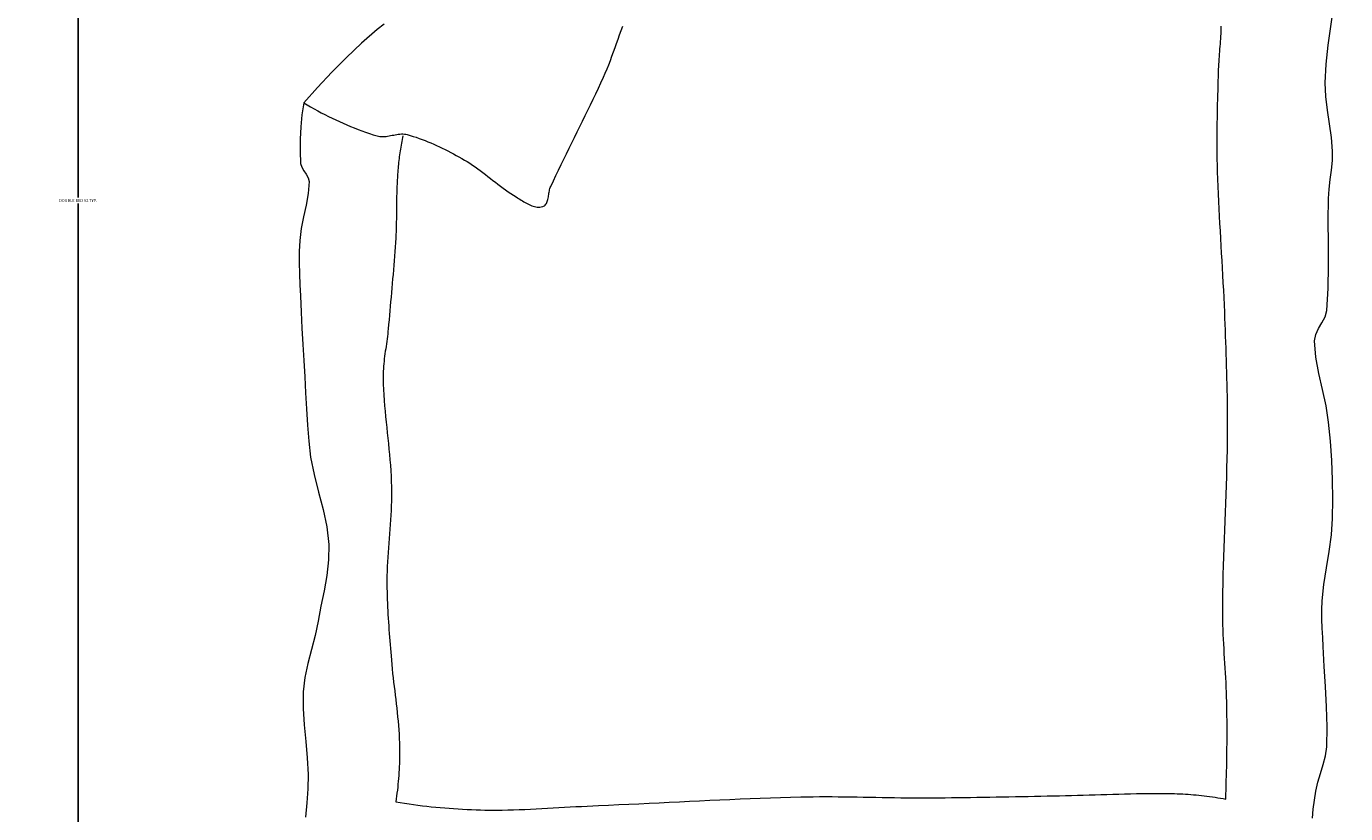
# Model space of a CAD drawing. Units: inches. Extents: x 1441 to 2460, y 1648 to 2683.
# Tile 23 of 35: x 1792 to 1874, y 2204 to 2253. Entities that reach past the tile are written whole.
import ezdxf

# ---------------------------------------------------------------- set-up
doc = ezdxf.new("R2010")
doc.units = ezdxf.units.IN
doc.layers.add('A-ANNO-DIMS', color=2, linetype='Continuous', lineweight=18)
doc.layers.add('A-FURN', color=8, linetype='Continuous', lineweight=15)
doc.styles.get("Standard").update_dxf_attribs({"font": 'arial.ttf'})
doc.dimstyles.get("Standard").update_dxf_attribs({"dimtxt": 0.18, "dimasz": 0.18, "dimexe": 0.18, "dimexo": 0.0625, "dimgap": 0.09, "dimtad": 0, "dimtih": 1, "dimtoh": 1, "dimdec": 4, "dimzin": 0, "dimdsep": 46, "dimtxsty": 'Standard', "dimcen": 0.09, "dimadec": 0, "dimazin": 0, "dimtfac": 1, "dimtdec": 4, "dimtofl": 0, "dimtmove": 0, "dimatfit": 3, "dimfxl": 1, "dimtolj": 1, "dimtzin": 0, "dimarcsym": 0})

# ---------------------------------------------------------------- blocks, each defined once
blk = doc.blocks.new('BED-DOUBLE-PLAN')
for p, q in [((64.222, 56.681), (64.382, 57.848)), ((5.285, 56.837), (4.851, 56.5)), ((20.05, 56.435), (20.15, 56.7)), ((57.394, 56.548), (57.398, 56.707)), ((64.06, 55.515), (64.222, 56.681)), ((4.851, 56.5), (3.888, 55.638)), ((19.761, 55.634), (19.856, 55.902)), ((19.856, 55.902), (19.952, 56.169)), ((19.952, 56.169), (20.05, 56.435)), ((57.353, 55.757), (57.363, 55.915)), ((57.363, 55.915), (57.373, 56.073)), ((57.373, 56.073), (57.382, 56.232)), ((57.382, 56.232), (57.389, 56.39)), ((57.389, 56.39), (57.394, 56.548)), ((3.888, 55.638), (2.949, 54.748)), ((19.474, 54.832), (19.571, 55.099)), ((19.571, 55.099), (19.666, 55.367)), ((19.666, 55.367), (19.761, 55.634)), ((57.291, 54.965), (57.304, 55.123)), ((57.304, 55.123), (57.316, 55.282)), ((57.316, 55.282), (57.329, 55.44)), ((57.329, 55.44), (57.341, 55.598)), ((57.341, 55.598), (57.353, 55.757)), ((63.929, 54.347), (64.06, 55.515)), ((2.949, 54.748), (2.036, 53.833)), ((19.169, 54.039), (19.274, 54.302)), ((19.274, 54.302), (19.375, 54.566)), ((19.375, 54.566), (19.474, 54.832)), ((57.239, 54.173), (57.247, 54.332)), ((57.247, 54.332), (57.257, 54.49)), ((57.257, 54.49), (57.268, 54.649)), ((57.268, 54.649), (57.279, 54.807)), ((57.279, 54.807), (57.291, 54.965)), ((63.863, 53.174), (63.929, 54.347)), ((2.036, 53.833), (1.148, 52.892)), ((18.788, 53.177), (18.945, 53.52)), ((18.945, 53.52), (19.059, 53.778)), ((19.059, 53.778), (19.169, 54.039)), ((57.21, 53.28), (57.218, 53.568)), ((57.218, 53.568), (57.227, 53.856)), ((57.227, 53.856), (57.232, 54.015)), ((57.232, 54.015), (57.239, 54.173)), ((1.148, 52.892), (0.288, 51.928)), ((18.468, 52.493), (18.629, 52.834)), ((18.629, 52.834), (18.788, 53.177)), ((57.186, 52.417), (57.194, 52.705)), ((57.194, 52.705), (57.202, 52.993)), ((57.202, 52.993), (57.21, 53.28)), ((63.897, 52.321), (63.863, 53.174)), ((0.288, 51.928), (0.178, 51.18)), ((0.288, 51.928), (0.502, 51.799)), ((0.502, 51.799), (0.719, 51.672)), ((17.979, 51.472), (18.143, 51.812)), ((18.143, 51.812), (18.306, 52.152)), ((18.306, 52.152), (18.468, 52.493)), ((57.164, 51.553), (57.171, 51.841)), ((57.171, 51.841), (57.178, 52.129)), ((57.178, 52.129), (57.186, 52.417)), ((64.002, 51.471), (63.897, 52.321)), ((0.178, 51.18), (0.104, 50.426)), ((0.719, 51.672), (0.936, 51.548)), ((0.936, 51.548), (1.156, 51.426)), ((1.156, 51.426), (1.377, 51.308)), ((1.377, 51.308), (1.6, 51.192)), ((1.6, 51.192), (1.824, 51.079)), ((1.824, 51.079), (2.05, 50.968)), ((2.05, 50.968), (2.277, 50.861)), ((17.648, 50.793), (17.814, 51.132)), ((17.814, 51.132), (17.979, 51.472)), ((57.147, 50.688), (57.152, 50.976)), ((57.152, 50.976), (57.158, 51.265)), ((57.158, 51.265), (57.164, 51.553)), ((64.135, 50.622), (64.002, 51.471)), ((0.104, 50.426), (0.065, 49.669)), ((2.277, 50.861), (2.505, 50.756)), ((2.505, 50.756), (2.735, 50.654)), ((2.735, 50.654), (2.966, 50.555)), ((2.966, 50.555), (3.198, 50.459)), ((3.198, 50.459), (3.432, 50.366)), ((3.432, 50.366), (3.666, 50.276)), ((3.666, 50.276), (3.901, 50.189)), ((3.901, 50.189), (4.138, 50.105)), ((4.138, 50.105), (4.375, 50.024)), ((17.147, 49.777), (17.314, 50.116)), ((17.314, 50.116), (17.481, 50.455)), ((17.481, 50.455), (17.648, 50.793)), ((57.138, 49.824), (57.14, 50.112)), ((57.14, 50.112), (57.143, 50.4)), ((57.143, 50.4), (57.147, 50.688)), ((64.256, 49.773), (64.135, 50.622)), ((0.065, 49.669), (0.062, 48.911)), ((4.375, 50.024), (4.613, 49.946)), ((4.613, 49.946), (4.852, 49.871)), ((4.852, 49.871), (4.943, 49.848)), ((4.943, 49.848), (5.034, 49.833)), ((5.034, 49.833), (5.127, 49.826)), ((5.127, 49.826), (5.22, 49.825)), ((5.22, 49.825), (5.314, 49.829)), ((5.314, 49.829), (5.409, 49.839)), ((5.409, 49.839), (5.504, 49.852)), ((5.504, 49.852), (5.6, 49.868)), ((5.6, 49.868), (5.695, 49.886)), ((5.695, 49.886), (5.791, 49.905)), ((5.791, 49.905), (5.887, 49.924)), ((5.887, 49.924), (5.983, 49.943)), ((5.983, 49.943), (6.079, 49.96)), ((6.079, 49.96), (6.174, 49.974)), ((6.174, 49.974), (6.269, 49.984)), ((6.269, 49.984), (6.363, 49.99)), ((6.347, 49.291), (6.326, 49.172)), ((6.368, 49.41), (6.347, 49.291)), ((6.363, 49.99), (6.457, 49.991)), ((6.39, 49.528), (6.368, 49.41)), ((6.412, 49.647), (6.39, 49.528)), ((6.436, 49.765), (6.412, 49.647)), ((6.46, 49.883), (6.436, 49.765)), ((6.457, 49.991), (6.55, 49.986)), ((6.55, 49.986), (6.643, 49.973)), ((6.643, 49.973), (6.734, 49.952)), ((6.734, 49.952), (6.921, 49.899)), ((6.921, 49.899), (7.107, 49.841)), ((7.107, 49.841), (7.292, 49.781)), ((7.292, 49.781), (7.476, 49.717)), ((7.476, 49.717), (7.659, 49.65)), ((7.659, 49.65), (7.841, 49.58)), ((7.841, 49.58), (8.022, 49.507)), ((8.022, 49.507), (8.202, 49.431)), ((8.202, 49.431), (8.381, 49.353)), ((8.381, 49.353), (8.56, 49.273)), ((8.56, 49.273), (8.737, 49.19)), ((16.813, 49.1), (16.98, 49.439)), ((16.98, 49.439), (17.147, 49.777)), ((57.137, 49.536), (57.138, 49.824)), ((57.137, 49.248), (57.137, 49.536)), ((64.322, 48.92), (64.256, 49.773)), ((0.062, 48.911), (0.095, 48.156)), ((6.221, 48.455), (6.207, 48.335)), ((6.237, 48.575), (6.221, 48.455)), ((6.253, 48.694), (6.237, 48.575)), ((6.27, 48.814), (6.253, 48.694)), ((6.288, 48.933), (6.27, 48.814)), ((6.307, 49.053), (6.288, 48.933)), ((6.326, 49.172), (6.307, 49.053)), ((8.737, 49.19), (8.913, 49.105)), ((8.913, 49.105), (9.088, 49.019)), ((9.088, 49.019), (9.263, 48.93)), ((9.263, 48.93), (9.436, 48.84)), ((9.436, 48.84), (9.609, 48.748)), ((9.609, 48.748), (9.781, 48.655)), ((9.781, 48.655), (9.952, 48.56)), ((9.952, 48.56), (10.122, 48.465)), ((10.122, 48.465), (10.291, 48.368)), ((16.481, 48.423), (16.647, 48.762)), ((16.647, 48.762), (16.813, 49.1)), ((57.139, 48.96), (57.137, 49.248)), ((57.142, 48.672), (57.139, 48.96)), ((57.147, 48.384), (57.142, 48.672)), ((64.311, 48.328), (64.322, 48.92)), ((0.095, 48.156), (0.161, 47.92)), ((0.161, 47.92), (0.294, 47.701)), ((0.294, 47.701), (0.446, 47.487)), ((6.146, 47.734), (6.136, 47.614)), ((6.156, 47.855), (6.146, 47.734)), ((6.168, 47.975), (6.156, 47.855)), ((6.18, 48.095), (6.168, 47.975)), ((6.193, 48.215), (6.18, 48.095)), ((6.207, 48.335), (6.193, 48.215)), ((10.291, 48.368), (10.462, 48.268)), ((10.462, 48.268), (10.629, 48.163)), ((10.629, 48.163), (10.794, 48.054)), ((10.794, 48.054), (10.957, 47.942)), ((10.957, 47.942), (11.118, 47.827)), ((11.118, 47.827), (11.277, 47.709)), ((11.277, 47.709), (11.435, 47.59)), ((15.987, 47.404), (16.151, 47.744)), ((16.151, 47.744), (16.315, 48.084)), ((16.315, 48.084), (16.481, 48.423)), ((57.153, 48.096), (57.147, 48.384)), ((57.167, 47.636), (57.153, 48.096)), ((57.182, 47.175), (57.167, 47.636)), ((64.185, 47.146), (64.258, 47.737)), ((64.258, 47.737), (64.311, 48.328)), ((0.446, 47.487), (0.571, 47.267)), ((0.62, 47.031), (0.562, 46.291)), ((0.571, 47.267), (0.62, 47.031)), ((6.095, 46.897), (6.087, 46.698)), ((6.104, 47.096), (6.095, 46.897)), ((6.114, 47.295), (6.104, 47.096)), ((6.127, 47.494), (6.114, 47.295)), ((6.136, 47.614), (6.127, 47.494)), ((11.435, 47.59), (11.593, 47.469)), ((11.593, 47.469), (11.749, 47.347)), ((11.749, 47.347), (11.905, 47.224)), ((11.905, 47.224), (12.061, 47.101)), ((12.061, 47.101), (12.218, 46.979)), ((12.218, 46.979), (12.374, 46.857)), ((12.374, 46.857), (12.532, 46.737)), ((15.663, 46.722), (15.824, 47.063)), ((15.824, 47.063), (15.987, 47.404)), ((57.2, 46.714), (57.182, 47.175)), ((64.117, 46.556), (64.185, 47.146)), ((0.562, 46.291), (0.434, 45.558)), ((6.072, 46.1), (6.069, 45.901)), ((6.076, 46.3), (6.072, 46.1)), ((6.081, 46.499), (6.076, 46.3)), ((6.087, 46.698), (6.081, 46.499)), ((12.532, 46.737), (12.691, 46.618)), ((12.691, 46.618), (12.851, 46.501)), ((12.851, 46.501), (13.012, 46.387)), ((13.012, 46.387), (13.176, 46.276)), ((13.176, 46.276), (13.342, 46.169)), ((13.342, 46.169), (13.511, 46.065)), ((13.511, 46.065), (13.587, 46.019)), ((13.587, 46.019), (13.664, 45.971)), ((15.486, 45.917), (15.502, 45.99)), ((15.502, 45.99), (15.515, 46.065)), ((15.515, 46.065), (15.527, 46.141)), ((15.527, 46.141), (15.539, 46.218)), ((15.539, 46.218), (15.551, 46.295)), ((15.551, 46.295), (15.564, 46.372)), ((15.564, 46.372), (15.578, 46.447)), ((15.578, 46.447), (15.595, 46.52)), ((15.595, 46.52), (15.614, 46.591)), ((15.614, 46.591), (15.636, 46.659)), ((15.636, 46.659), (15.663, 46.722)), ((57.22, 46.253), (57.2, 46.714)), ((57.241, 45.792), (57.22, 46.253)), ((64.074, 45.964), (64.117, 46.556)), ((0.434, 45.558), (0.277, 44.827)), ((6.062, 45.303), (6.06, 45.104)), ((6.064, 45.502), (6.062, 45.303)), ((6.067, 45.702), (6.064, 45.502)), ((6.069, 45.901), (6.067, 45.702)), ((13.664, 45.971), (13.742, 45.922)), ((13.742, 45.922), (13.822, 45.871)), ((13.822, 45.871), (13.902, 45.821)), ((13.902, 45.821), (13.983, 45.771)), ((13.983, 45.771), (14.065, 45.723)), ((14.065, 45.723), (14.147, 45.676)), ((14.147, 45.676), (14.231, 45.631)), ((14.231, 45.631), (14.314, 45.589)), ((14.314, 45.589), (14.398, 45.551)), ((14.398, 45.551), (14.483, 45.517)), ((14.483, 45.517), (14.567, 45.487)), ((14.567, 45.487), (14.652, 45.463)), ((14.652, 45.463), (14.737, 45.445)), ((14.737, 45.445), (14.822, 45.434)), ((14.822, 45.434), (14.907, 45.429)), ((14.907, 45.429), (14.992, 45.433)), ((14.992, 45.433), (15.076, 45.445)), ((15.076, 45.445), (15.16, 45.466)), ((15.16, 45.466), (15.221, 45.49)), ((15.221, 45.49), (15.274, 45.522)), ((15.274, 45.522), (15.32, 45.561)), ((15.32, 45.561), (15.36, 45.608)), ((15.36, 45.608), (15.394, 45.66)), ((15.394, 45.66), (15.423, 45.718)), ((15.423, 45.718), (15.448, 45.78)), ((15.448, 45.78), (15.468, 45.847)), ((15.468, 45.847), (15.486, 45.917)), ((57.264, 45.332), (57.241, 45.792)), ((57.289, 44.871), (57.264, 45.332)), ((64.052, 44.569), (64.074, 45.964)), ((0.277, 44.827), (0.13, 44.094)), ((6.05, 44.506), (6.045, 44.306)), ((6.054, 44.705), (6.05, 44.506)), ((6.057, 44.904), (6.054, 44.705)), ((6.06, 45.104), (6.057, 44.904)), ((57.314, 44.411), (57.289, 44.871)), ((57.34, 43.95), (57.314, 44.411)), ((64.063, 43.173), (64.052, 44.569)), ((0.13, 44.094), (0.035, 43.356)), ((6.022, 43.709), (6.011, 43.51)), ((6.031, 43.908), (6.022, 43.709)), ((6.039, 44.107), (6.031, 43.908)), ((6.045, 44.306), (6.039, 44.107)), ((57.367, 43.49), (57.34, 43.95)), ((0.035, 43.356), (0.002, 42.668)), ((5.975, 42.943), (5.955, 42.66)), ((5.993, 43.227), (5.975, 42.943)), ((6.011, 43.51), (5.993, 43.227)), ((57.394, 43.029), (57.367, 43.49)), ((57.42, 42.569), (57.394, 43.029)), ((64.074, 41.778), (64.063, 43.173)), ((0.002, 42.668), (0.002, 41.978)), ((0.002, 41.978), (0.023, 41.288)), ((5.914, 42.093), (5.892, 41.81)), ((5.935, 42.376), (5.914, 42.093)), ((5.955, 42.66), (5.935, 42.376)), ((57.447, 42.108), (57.42, 42.569)), ((57.474, 41.648), (57.447, 42.108)), ((0.023, 41.288), (0.053, 40.599)), ((5.846, 41.243), (5.822, 40.96)), ((5.869, 41.527), (5.846, 41.243)), ((5.892, 41.81), (5.869, 41.527)), ((57.499, 41.187), (57.474, 41.648)), ((57.524, 40.727), (57.499, 41.187)), ((64.051, 40.384), (64.074, 41.778)), ((0.053, 40.599), (0.083, 39.909)), ((5.774, 40.394), (5.749, 40.111)), ((5.798, 40.677), (5.774, 40.394)), ((5.822, 40.96), (5.798, 40.677)), ((57.548, 40.266), (57.524, 40.727)), ((57.57, 39.806), (57.548, 40.266)), ((63.96, 38.994), (64.051, 40.384)), ((0.083, 39.909), (0.124, 38.9)), ((5.698, 39.545), (5.673, 39.262)), ((5.724, 39.828), (5.698, 39.545)), ((5.749, 40.111), (5.724, 39.828)), ((57.59, 39.345), (57.57, 39.806)), ((0.124, 38.9), (0.172, 37.892)), ((5.621, 38.696), (5.596, 38.413)), ((5.647, 38.979), (5.621, 38.696)), ((5.673, 39.262), (5.647, 38.979)), ((57.609, 38.884), (57.59, 39.345)), ((57.623, 38.511), (57.609, 38.884)), ((63.663, 38.235), (63.855, 38.605)), ((63.855, 38.605), (63.96, 38.994)), ((0.172, 37.892), (0.227, 36.884)), ((5.545, 37.847), (5.53, 37.692)), ((5.57, 38.13), (5.545, 37.847)), ((5.596, 38.413), (5.57, 38.13)), ((57.637, 38.138), (57.623, 38.511)), ((57.652, 37.765), (57.637, 38.138)), ((63.274, 37.501), (63.447, 37.871)), ((63.447, 37.871), (63.663, 38.235)), ((5.453, 37.073), (5.432, 36.918)), ((5.474, 37.227), (5.453, 37.073)), ((5.494, 37.382), (5.474, 37.227)), ((5.513, 37.537), (5.494, 37.382)), ((5.53, 37.692), (5.513, 37.537)), ((57.666, 37.393), (57.652, 37.765)), ((57.68, 37.02), (57.666, 37.393)), ((57.693, 36.647), (57.68, 37.02)), ((63.206, 37.11), (63.274, 37.501)), ((63.291, 36.09), (63.206, 37.11)), ((0.227, 36.884), (0.286, 35.876)), ((5.324, 36.144), (5.304, 35.989)), ((5.344, 36.299), (5.324, 36.144)), ((5.366, 36.454), (5.344, 36.299)), ((5.388, 36.608), (5.366, 36.454)), ((5.41, 36.763), (5.388, 36.608)), ((5.432, 36.918), (5.41, 36.763)), ((57.706, 36.274), (57.693, 36.647)), ((57.718, 35.901), (57.706, 36.274)), ((0.286, 35.876), (0.348, 34.868)), ((5.245, 35.369), (5.236, 35.214)), ((5.256, 35.524), (5.245, 35.369)), ((5.27, 35.679), (5.256, 35.524)), ((5.287, 35.834), (5.27, 35.679)), ((5.304, 35.989), (5.287, 35.834)), ((57.73, 35.528), (57.718, 35.901)), ((57.741, 35.155), (57.73, 35.528)), ((63.474, 35.079), (63.291, 36.09)), ((0.348, 34.868), (0.404, 33.866)), ((5.23, 35.059), (5.228, 34.903)), ((5.228, 34.903), (5.229, 34.747)), ((5.229, 34.747), (5.239, 34.409)), ((5.236, 35.214), (5.23, 35.059)), ((57.751, 34.782), (57.741, 35.155)), ((57.761, 34.409), (57.751, 34.782)), ((63.703, 34.073), (63.474, 35.079)), ((0.404, 33.866), (0.456, 32.863)), ((5.239, 34.409), (5.254, 34.072)), ((5.254, 34.072), (5.274, 33.735)), ((5.274, 33.735), (5.297, 33.397)), ((57.769, 34.036), (57.761, 34.409)), ((57.776, 33.663), (57.769, 34.036)), ((63.921, 33.064), (63.703, 34.073)), ((0.456, 32.863), (0.516, 31.861)), ((5.297, 33.397), (5.324, 33.06)), ((5.324, 33.06), (5.354, 32.724)), ((57.782, 33.29), (57.776, 33.663)), ((57.787, 32.917), (57.782, 33.29)), ((57.79, 32.543), (57.787, 32.917)), ((64.075, 32.048), (63.921, 33.064)), ((5.354, 32.724), (5.386, 32.387)), ((5.386, 32.387), (5.42, 32.05)), ((5.42, 32.05), (5.455, 31.714)), ((57.792, 32.17), (57.79, 32.543)), ((57.792, 31.797), (57.792, 32.17)), ((64.186, 30.851), (64.075, 32.048)), ((0.516, 31.861), (0.599, 30.861)), ((5.455, 31.714), (5.491, 31.377)), ((5.491, 31.377), (5.526, 31.04)), ((57.785, 30.869), (57.79, 31.424)), ((57.79, 31.424), (57.792, 31.797)), ((0.599, 30.861), (0.719, 29.866)), ((5.526, 31.04), (5.561, 30.704)), ((5.561, 30.704), (5.595, 30.367)), ((57.777, 30.314), (57.785, 30.869)), ((64.273, 29.652), (64.186, 30.851)), ((0.719, 29.866), (0.929, 28.772)), ((5.595, 30.367), (5.627, 30.03)), ((5.627, 30.03), (5.656, 29.694)), ((5.656, 29.694), (5.683, 29.357)), ((57.751, 29.204), (57.765, 29.759)), ((57.765, 29.759), (57.777, 30.314)), ((64.329, 28.45), (64.273, 29.652)), ((0.929, 28.772), (1.205, 27.689)), ((5.683, 29.357), (5.706, 29.019)), ((5.706, 29.019), (5.725, 28.682)), ((57.735, 28.65), (57.751, 29.204)), ((5.725, 28.682), (5.74, 28.344)), ((5.74, 28.344), (5.749, 28.007)), ((5.749, 28.007), (5.752, 27.715)), ((57.698, 27.54), (57.718, 28.095)), ((57.718, 28.095), (57.735, 28.65)), ((64.349, 27.249), (64.329, 28.45)), ((1.205, 27.689), (1.489, 26.608)), ((5.744, 27.131), (5.734, 26.839)), ((5.75, 27.423), (5.744, 27.131)), ((5.752, 27.715), (5.75, 27.423)), ((57.678, 26.985), (57.698, 27.54)), ((64.328, 26.047), (64.349, 27.249)), ((1.489, 26.608), (1.722, 25.521)), ((5.72, 26.547), (5.704, 26.255)), ((5.734, 26.839), (5.72, 26.547)), ((57.636, 25.876), (57.657, 26.431)), ((57.657, 26.431), (57.678, 26.985)), ((1.722, 25.521), (1.846, 24.419)), ((5.666, 25.672), (5.644, 25.38)), ((5.686, 25.964), (5.666, 25.672)), ((5.704, 26.255), (5.686, 25.964)), ((57.615, 25.321), (57.636, 25.876)), ((64.248, 25.017), (64.328, 26.047)), ((5.6, 24.797), (5.577, 24.505)), ((5.622, 25.089), (5.6, 24.797)), ((5.644, 25.38), (5.622, 25.089)), ((57.575, 24.212), (57.595, 24.766)), ((57.595, 24.766), (57.615, 25.321)), ((64.106, 23.991), (64.248, 25.017)), ((1.846, 24.419), (1.831, 23.458)), ((5.535, 23.922), (5.516, 23.63)), ((5.556, 24.214), (5.535, 23.922)), ((5.577, 24.505), (5.556, 24.214)), ((57.556, 23.657), (57.575, 24.212)), ((63.939, 22.967), (64.106, 23.991)), ((1.831, 23.458), (1.723, 22.5)), ((5.485, 23.047), (5.475, 22.755)), ((5.499, 23.338), (5.485, 23.047)), ((5.516, 23.63), (5.499, 23.338)), ((57.525, 22.547), (57.54, 23.102)), ((57.54, 23.102), (57.556, 23.657)), ((1.723, 22.5), (1.555, 21.544)), ((5.467, 22.463), (5.464, 22.171)), ((5.464, 22.171), (5.465, 21.936)), ((5.475, 22.755), (5.467, 22.463)), ((57.512, 21.992), (57.525, 22.547)), ((63.782, 21.942), (63.939, 22.967)), ((1.555, 21.544), (1.362, 20.592)), ((5.465, 21.936), (5.467, 21.701)), ((5.467, 21.701), (5.472, 21.467)), ((5.472, 21.467), (5.478, 21.232)), ((57.495, 20.882), (57.502, 21.437)), ((57.502, 21.437), (57.512, 21.992)), ((63.671, 20.913), (63.782, 21.942)), ((1.362, 20.592), (1.181, 19.64)), ((5.478, 21.232), (5.486, 20.998)), ((5.486, 20.998), (5.495, 20.763)), ((5.495, 20.763), (5.506, 20.529)), ((5.506, 20.529), (5.518, 20.295)), ((57.492, 20.327), (57.495, 20.882)), ((63.649, 20.346), (63.671, 20.913)), ((5.518, 20.295), (5.531, 20.06)), ((5.531, 20.06), (5.546, 19.826)), ((5.546, 19.826), (5.561, 19.592)), ((57.493, 20.027), (57.492, 20.327)), ((57.497, 19.727), (57.493, 20.027)), ((57.504, 19.427), (57.497, 19.727)), ((63.657, 19.777), (63.649, 20.346)), ((63.683, 19.209), (63.657, 19.777)), ((1.181, 19.64), (0.996, 18.76)), ((5.561, 19.592), (5.577, 19.358)), ((5.577, 19.358), (5.594, 19.123)), ((5.594, 19.123), (5.612, 18.889)), ((5.612, 18.889), (5.629, 18.655)), ((57.513, 19.127), (57.504, 19.427)), ((57.525, 18.827), (57.513, 19.127)), ((63.715, 18.64), (63.683, 19.209)), ((0.996, 18.76), (0.773, 17.887)), ((5.629, 18.655), (5.647, 18.421)), ((5.647, 18.421), (5.666, 18.187)), ((5.666, 18.187), (5.684, 17.953)), ((57.538, 18.527), (57.525, 18.827)), ((57.554, 18.227), (57.538, 18.527)), ((57.57, 17.927), (57.554, 18.227)), ((63.74, 18.071), (63.715, 18.64)), ((63.8, 16.821), (63.74, 18.071)), ((0.773, 17.887), (0.551, 17.013)), ((5.684, 17.953), (5.702, 17.719)), ((5.702, 17.719), (5.721, 17.485)), ((5.721, 17.485), (5.743, 17.213)), ((57.587, 17.627), (57.57, 17.927)), ((57.605, 17.327), (57.587, 17.627)), ((57.623, 17.027), (57.605, 17.327)), ((0.551, 17.013), (0.366, 16.135)), ((5.743, 17.213), (5.768, 16.942)), ((5.768, 16.942), (5.794, 16.671)), ((5.794, 16.671), (5.823, 16.399)), ((57.641, 16.727), (57.623, 17.027)), ((57.659, 16.427), (57.641, 16.727)), ((57.676, 16.127), (57.659, 16.427)), ((63.878, 15.571), (63.8, 16.821)), ((0.366, 16.135), (0.257, 15.246)), ((5.823, 16.399), (5.853, 16.128)), ((5.853, 16.128), (5.884, 15.857)), ((5.884, 15.857), (5.916, 15.587)), ((57.692, 15.827), (57.676, 16.127)), ((57.706, 15.527), (57.692, 15.827)), ((0.257, 15.246), (0.244, 14.217)), ((5.916, 15.587), (5.948, 15.316)), ((5.948, 15.316), (5.981, 15.045)), ((5.981, 15.045), (6.013, 14.774)), ((57.719, 15.227), (57.706, 15.527)), ((57.73, 14.927), (57.719, 15.227)), ((57.739, 14.627), (57.73, 14.927)), ((63.95, 14.321), (63.878, 15.571)), ((0.244, 14.217), (0.31, 13.189)), ((6.013, 14.774), (6.044, 14.503)), ((6.044, 14.503), (6.075, 14.232)), ((6.075, 14.232), (6.104, 13.961)), ((6.104, 13.961), (6.131, 13.69)), ((57.745, 14.327), (57.739, 14.627)), ((57.749, 14.039), (57.745, 14.327)), ((57.752, 13.751), (57.749, 14.039)), ((63.987, 13.071), (63.95, 14.321)), ((0.31, 13.189), (0.413, 12.16)), ((6.131, 13.69), (6.157, 13.419)), ((6.157, 13.419), (6.18, 13.147)), ((6.18, 13.147), (6.201, 12.876)), ((57.754, 13.463), (57.752, 13.751)), ((57.756, 13.174), (57.754, 13.463)), ((57.757, 12.886), (57.756, 13.174)), ((6.201, 12.876), (6.219, 12.604)), ((6.219, 12.604), (6.233, 12.332)), ((6.233, 12.332), (6.244, 12.06)), ((57.756, 12.31), (57.757, 12.598)), ((57.757, 12.598), (57.757, 12.886)), ((63.964, 11.821), (63.987, 13.071)), ((0.413, 12.16), (0.51, 11.13)), ((6.244, 12.06), (6.249, 11.876)), ((6.249, 11.876), (6.252, 11.692)), ((6.252, 11.692), (6.254, 11.508)), ((6.254, 11.508), (6.253, 11.324)), ((57.749, 11.446), (57.752, 11.734)), ((57.752, 11.734), (57.754, 12.022)), ((57.754, 12.022), (57.756, 12.31)), ((63.889, 11.262), (63.964, 11.821)), ((0.51, 11.13), (0.56, 10.1)), ((6.242, 10.772), (6.235, 10.588)), ((6.248, 10.956), (6.242, 10.772)), ((6.251, 11.14), (6.248, 10.956)), ((6.253, 11.324), (6.251, 11.14)), ((57.734, 10.582), (57.74, 10.87)), ((57.74, 10.87), (57.744, 11.158)), ((57.744, 11.158), (57.749, 11.446)), ((63.572, 10.169), (63.745, 10.713)), ((63.745, 10.713), (63.889, 11.262)), ((0.56, 10.1), (0.539, 9.213)), ((6.189, 9.854), (6.173, 9.67)), ((6.203, 10.037), (6.189, 9.854)), ((6.215, 10.221), (6.203, 10.037)), ((6.226, 10.405), (6.215, 10.221)), ((6.235, 10.588), (6.226, 10.405)), ((57.712, 9.718), (57.72, 10.006)), ((57.72, 10.006), (57.727, 10.294)), ((57.727, 10.294), (57.734, 10.582)), ((63.406, 9.622), (63.572, 10.169)), ((0.539, 9.213), (0.478, 8.327)), ((6.115, 9.121), (6.092, 8.939)), ((6.136, 9.304), (6.115, 9.121)), ((6.155, 9.487), (6.136, 9.304)), ((6.173, 9.67), (6.155, 9.487)), ((57.683, 8.855), (57.694, 9.142)), ((57.694, 9.142), (57.703, 9.43)), ((57.703, 9.43), (57.712, 9.718)), ((63.198, 8.508), (63.284, 9.068)), ((63.284, 9.068), (63.406, 9.622)), ((0.478, 8.327), (0.407, 7.441)), ((6.041, 8.575), (6.013, 8.393)), ((6.013, 8.393), (6.289, 8.349)), ((6.067, 8.756), (6.041, 8.575)), ((6.092, 8.939), (6.067, 8.756)), ((6.289, 8.349), (6.564, 8.306)), ((6.564, 8.306), (6.841, 8.266)), ((6.841, 8.266), (7.117, 8.228)), ((7.117, 8.228), (7.394, 8.191)), ((19.266, 8.194), (19.895, 8.222)), ((19.895, 8.222), (20.525, 8.251)), ((20.525, 8.251), (21.154, 8.28)), ((21.154, 8.28), (21.783, 8.311)), ((21.783, 8.311), (22.412, 8.341)), ((22.412, 8.341), (23.042, 8.372)), ((23.042, 8.372), (23.671, 8.403)), ((23.671, 8.403), (24.3, 8.434)), ((24.3, 8.434), (24.929, 8.464)), ((24.929, 8.464), (25.559, 8.494)), ((25.559, 8.494), (26.188, 8.523)), ((26.188, 8.523), (26.817, 8.551)), ((26.817, 8.551), (27.447, 8.578)), ((27.447, 8.578), (28.076, 8.604)), ((28.076, 8.604), (28.705, 8.628)), ((28.705, 8.628), (29.335, 8.65)), ((29.335, 8.65), (29.964, 8.67)), ((29.964, 8.67), (30.594, 8.689)), ((30.594, 8.689), (31.224, 8.705)), ((31.224, 8.705), (31.613, 8.712)), ((31.613, 8.712), (32.002, 8.718)), ((32.002, 8.718), (32.391, 8.72)), ((32.391, 8.72), (32.781, 8.721)), ((32.781, 8.721), (33.17, 8.72)), ((33.17, 8.72), (33.559, 8.717)), ((33.559, 8.717), (33.948, 8.713)), ((33.948, 8.713), (34.338, 8.707)), ((34.338, 8.707), (34.727, 8.701)), ((34.727, 8.701), (35.116, 8.694)), ((35.116, 8.694), (35.506, 8.687)), ((35.506, 8.687), (35.895, 8.679)), ((35.895, 8.679), (36.284, 8.672)), ((36.284, 8.672), (36.674, 8.665)), ((36.674, 8.665), (37.063, 8.659)), ((37.063, 8.659), (37.452, 8.653)), ((37.452, 8.653), (37.841, 8.649)), ((37.841, 8.649), (38.231, 8.646)), ((38.231, 8.646), (38.62, 8.645)), ((38.62, 8.645), (39.009, 8.645)), ((39.009, 8.645), (39.407, 8.647)), ((39.407, 8.647), (39.805, 8.65)), ((39.805, 8.65), (40.203, 8.654)), ((40.203, 8.654), (40.601, 8.658)), ((40.601, 8.658), (40.999, 8.663)), ((40.999, 8.663), (41.397, 8.668)), ((41.397, 8.668), (41.795, 8.674)), ((41.795, 8.674), (42.193, 8.68)), ((42.193, 8.68), (42.591, 8.687)), ((42.591, 8.687), (42.989, 8.694)), ((42.989, 8.694), (43.387, 8.701)), ((43.387, 8.701), (43.785, 8.708)), ((43.785, 8.708), (44.183, 8.716)), ((44.183, 8.716), (44.581, 8.723)), ((44.581, 8.723), (44.979, 8.731)), ((44.979, 8.731), (45.376, 8.739)), ((45.376, 8.739), (45.774, 8.746)), ((45.774, 8.746), (46.172, 8.754)), ((46.172, 8.754), (46.57, 8.761)), ((46.57, 8.761), (46.968, 8.768)), ((46.968, 8.768), (47.336, 8.775)), ((47.336, 8.775), (47.704, 8.784)), ((47.704, 8.784), (48.071, 8.793)), ((48.071, 8.793), (48.439, 8.804)), ((48.439, 8.804), (48.807, 8.815)), ((48.807, 8.815), (49.174, 8.827)), ((49.174, 8.827), (49.542, 8.839)), ((49.542, 8.839), (49.91, 8.85)), ((49.91, 8.85), (50.278, 8.862)), ((50.278, 8.862), (50.645, 8.873)), ((50.645, 8.873), (51.013, 8.884)), ((51.013, 8.884), (51.381, 8.893)), ((51.381, 8.893), (51.748, 8.902)), ((51.748, 8.902), (52.116, 8.909)), ((52.116, 8.909), (52.484, 8.915)), ((52.484, 8.915), (52.851, 8.919)), ((52.851, 8.919), (53.219, 8.92)), ((53.219, 8.92), (53.587, 8.92)), ((53.587, 8.92), (53.955, 8.917)), ((53.955, 8.917), (54.322, 8.912)), ((54.322, 8.912), (54.491, 8.908)), ((54.491, 8.908), (54.659, 8.902)), ((54.659, 8.902), (54.827, 8.896)), ((54.827, 8.896), (54.996, 8.888)), ((54.996, 8.888), (55.164, 8.878)), ((55.164, 8.878), (55.332, 8.867)), ((55.332, 8.867), (55.5, 8.855)), ((55.5, 8.855), (55.668, 8.841)), ((55.668, 8.841), (55.836, 8.826)), ((55.836, 8.826), (56.004, 8.809)), ((56.004, 8.809), (56.172, 8.791)), ((56.172, 8.791), (56.339, 8.772)), ((56.339, 8.772), (56.507, 8.751)), ((56.507, 8.751), (56.674, 8.729)), ((56.674, 8.729), (56.841, 8.705)), ((56.841, 8.705), (57.008, 8.68)), ((57.008, 8.68), (57.174, 8.654)), ((57.174, 8.654), (57.34, 8.626)), ((57.34, 8.626), (57.506, 8.597)), ((57.506, 8.597), (57.672, 8.567)), ((57.672, 8.567), (57.683, 8.855)), ((63.122, 7.945), (63.198, 8.508)), ((7.394, 8.191), (7.671, 8.157)), ((7.671, 8.157), (7.949, 8.125)), ((7.949, 8.125), (8.226, 8.094)), ((8.226, 8.094), (8.504, 8.066)), ((8.504, 8.066), (8.783, 8.04)), ((8.783, 8.04), (9.061, 8.016)), ((9.061, 8.016), (9.339, 7.993)), ((9.339, 7.993), (9.618, 7.973)), ((9.618, 7.973), (9.897, 7.955)), ((9.897, 7.955), (10.175, 7.939)), ((10.175, 7.939), (10.454, 7.925)), ((10.454, 7.925), (10.733, 7.913)), ((10.733, 7.913), (11.012, 7.903)), ((11.012, 7.903), (11.291, 7.894)), ((11.291, 7.894), (11.57, 7.888)), ((11.57, 7.888), (11.924, 7.884)), ((11.924, 7.884), (12.277, 7.883)), ((12.277, 7.883), (12.631, 7.886)), ((12.631, 7.886), (12.984, 7.892)), ((12.984, 7.892), (13.338, 7.9)), ((13.338, 7.9), (13.691, 7.912)), ((13.691, 7.912), (14.044, 7.925)), ((14.044, 7.925), (14.397, 7.94)), ((14.397, 7.94), (14.751, 7.957)), ((14.751, 7.957), (15.104, 7.975)), ((15.104, 7.975), (15.457, 7.995)), ((15.457, 7.995), (15.811, 8.015)), ((15.811, 8.015), (16.164, 8.035)), ((16.164, 8.035), (16.517, 8.056)), ((16.517, 8.056), (16.87, 8.076)), ((16.87, 8.076), (17.224, 8.097)), ((17.224, 8.097), (17.577, 8.116)), ((17.577, 8.116), (17.93, 8.134)), ((17.93, 8.134), (18.283, 8.152)), ((18.283, 8.152), (18.637, 8.167)), ((18.637, 8.167), (19.266, 8.194)), ((63.071, 7.38), (63.122, 7.945))]:
    blk.add_line(p, q)
blk = doc.blocks.new('*D22')
at = {"layer": 'A-ANNO-DIMS', "color": 0, "lineweight": -2, "transparency": 16777216}
for p, q in [((1809.14, 2287.87), (1795.269, 2287.87)), ((1795.449, 2287.69), (1795.449, 2242.209)), ((1795.449, 2196.362), (1795.449, 2241.843)), ((1809.14, 2196.182), (1795.269, 2196.182))]:
    blk.add_line(p, q, dxfattribs=at)
at = {"layer": 'A-ANNO-DIMS', "color": 0, "transparency": 16777216}
for points in [[(1795.419, 2287.69), (1795.479, 2287.69), (1795.449, 2287.87)], [(1795.419, 2196.362), (1795.479, 2196.362), (1795.449, 2196.182)]]:
    blk.add_solid(points, dxfattribs=at)
at = {"layer": 'Defpoints', "color": 0, "transparency": 16777216}
for p in [(1795.449, 2287.87), (1809.202, 2287.87), (1809.202, 2196.182)]:
    blk.add_point(p, dxfattribs=at)
at = {"layer": 'A-ANNO-DIMS', "color": 0, "transparency": 16777216, "insert": (1795.449, 2242.026), "char_height": 0.18, "attachment_point": 5}
blk.add_mtext('\\A1;DOUBLE BED 92 TYP.', dxfattribs=at)
blk = doc.blocks.new('*D67')
at = {"layer": 'A-ANNO-DIMS', "color": 0, "lineweight": -2, "transparency": 16777216}
for p, q in [((1889.448, 2298.695), (1916.216, 2298.695)), ((1916.036, 2298.515), (1916.036, 2055.938)), ((1916.036, 1812.997), (1916.036, 2055.574)), ((1758.224, 1812.817), (1916.216, 1812.817))]:
    blk.add_line(p, q, dxfattribs=at)
at = {"layer": 'A-ANNO-DIMS', "color": 0, "transparency": 16777216}
for points in [[(1916.006, 2298.515), (1916.066, 2298.515), (1916.036, 2298.695)], [(1916.006, 1812.997), (1916.066, 1812.997), (1916.036, 1812.817)]]:
    blk.add_solid(points, dxfattribs=at)
at = {"layer": 'Defpoints', "color": 0, "transparency": 16777216}
for p in [(1889.386, 2298.695), (1916.036, 2298.695), (1758.161, 1812.817)]:
    blk.add_point(p, dxfattribs=at)
at = {"layer": 'A-ANNO-DIMS', "color": 0, "transparency": 16777216, "insert": (1916.036, 2055.756), "char_height": 0.18, "attachment_point": 5}
blk.add_mtext('\\A1;485.9', dxfattribs=at)

msp = doc.modelspace()

# ---------------------------------------------------------------- block references
at = {"layer": 'A-FURN'}
msp.add_blockref('BED-DOUBLE-PLAN', (1809.2, 2196.18), dxfattribs=at)

# ---------------------------------------------------------------- dimensions: what is measured, and where the dimension line sits
at = {"layer": 'A-ANNO-DIMS'}
dim = msp.add_linear_dim(base=(1916.0359, 2298.6952), p1=(1758.1615, 1812.8171), p2=(1889.3859, 2298.6952), angle=90, dimstyle='Standard', override={"dimdec": 1, "dimlfac": 1, "dimrnd": 0, "dimzin": 0, "dimdsep": 46, "dimlunit": 2}, dxfattribs=at)
dim.commit()
dim.dimension.update_dxf_attribs({"geometry": '*D67', "text_midpoint": (1916.0359, 2055.7561)})
dim = msp.add_linear_dim(base=(1795.4489, 2287.8701), p1=(1809.2021, 2196.1822), p2=(1809.2021, 2287.8701), angle=90, text='DOUBLE BED <> TYP.', dimstyle='Standard', override={"dimdec": 0, "dimlfac": 1, "dimrnd": 0, "dimzin": 0, "dimdsep": 46, "dimlunit": 2}, dxfattribs=at)
dim.commit()
dim.dimension.update_dxf_attribs({"geometry": '*D22', "text_midpoint": (1795.4489, 2242.0262)})

doc.saveas('drawing.dxf')
